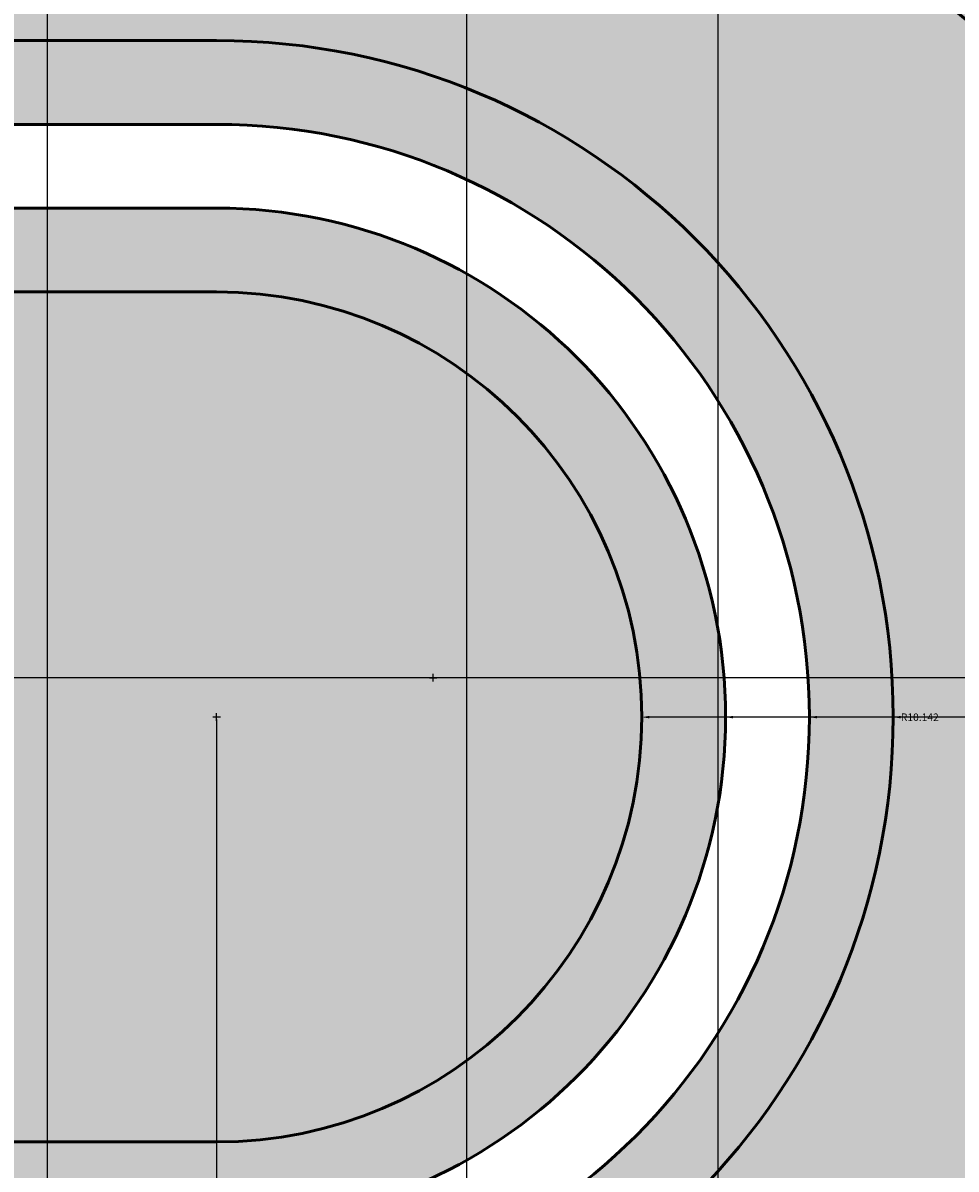
# Model space of a CAD drawing. Units: inches. Extents: x -12 to 334, y -10 to 186.
# Tile 54 of 77: x 222 to 244, y 69 to 96. Entities that reach past the tile are written whole.
import ezdxf

# ---------------------------------------------------------------- set-up
doc = ezdxf.new("R2010")
doc.units = ezdxf.units.IN
doc.header["$MEASUREMENT"] = 0
for name, color, linetype, lineweight in [('M-DIMS', 2, 'Continuous', 18), ('M-EQPM', 7, 'Continuous', 50), ('M-EQPM-PATT', 8, 'Continuous', 18)]:
    doc.layers.add(name, color=color, linetype=linetype, lineweight=lineweight)
doc.styles.get("Standard").update_dxf_attribs({"font": 'arial.ttf'})
doc.dimstyles.get("Standard").update_dxf_attribs({"dimtxt": 0.18, "dimasz": 0.18, "dimexe": 0.18, "dimexo": 0.0625, "dimgap": 0.09, "dimtad": 0, "dimtih": 1, "dimtoh": 1, "dimdec": 4, "dimzin": 0, "dimdsep": 46, "dimtxsty": 'Standard', "dimcen": 0.09, "dimadec": 0, "dimazin": 0, "dimtfac": 1, "dimtdec": 4, "dimtofl": 0, "dimtmove": 0, "dimatfit": 3, "dimfxl": 1, "dimtolj": 1, "dimtzin": 0, "dimarcsym": 0})

# ---------------------------------------------------------------- blocks, each defined once
blk = doc.blocks.new('*D1')
at = {"layer": 'Defpoints', "color": 0, "transparency": 16777216}
for p in [(281.426, 91.899), (3.376, 80.692), (281.426, 14.304)]:
    blk.add_point(p, dxfattribs=at)
at = {"layer": 'M-DIMS', "color": 0, "lineweight": -2, "transparency": 16777216}
for p, q in [((281.426, 91.836), (281.426, 14.124)), ((3.376, 80.629), (3.376, 14.124)), ((3.556, 14.304), (141.935, 14.304)), ((281.246, 14.304), (142.867, 14.304))]:
    blk.add_line(p, q, dxfattribs=at)
at = {"layer": 'M-DIMS', "color": 0, "transparency": 16777216}
for points in [[(3.556, 14.334), (3.556, 14.274), (3.376, 14.304)], [(281.246, 14.334), (281.246, 14.274), (281.426, 14.304)]]:
    blk.add_solid(points, dxfattribs=at)
at = {"layer": 'M-DIMS', "color": 0, "transparency": 16777216, "insert": (142.401, 14.304), "char_height": 0.18, "attachment_point": 5}
blk.add_mtext('\\A1;278.05', dxfattribs=at)
blk = doc.blocks.new('*D17')
at = {"layer": 'Defpoints', "color": 0, "transparency": 16777216}
for p in [(106.177, 102.896), (105.892, 56.321), (295.976, 56.321)]:
    blk.add_point(p, dxfattribs=at)
at = {"layer": 'M-DIMS', "color": 0, "lineweight": -2, "transparency": 16777216}
for p, q in [((106.24, 102.896), (296.156, 102.896)), ((295.976, 102.716), (295.976, 79.79)), ((295.976, 56.501), (295.976, 79.426)), ((105.954, 56.321), (296.156, 56.321))]:
    blk.add_line(p, q, dxfattribs=at)
at = {"layer": 'M-DIMS', "color": 0, "transparency": 16777216}
for points in [[(295.946, 102.716), (296.006, 102.716), (295.976, 102.896)], [(295.946, 56.501), (296.006, 56.501), (295.976, 56.321)]]:
    blk.add_solid(points, dxfattribs=at)
at = {"layer": 'M-DIMS', "color": 0, "transparency": 16777216, "insert": (295.976, 79.608), "char_height": 0.18, "attachment_point": 5}
blk.add_mtext('\\A1;46.575', dxfattribs=at)
blk = doc.blocks.new('*D27')
at = {"layer": 'Defpoints', "color": 0, "transparency": 16777216}
for p in [(238.576, 169.385), (216.576, 32.854), (238.576, 32.854)]:
    blk.add_point(p, dxfattribs=at)
at = {"layer": 'M-DIMS', "color": 0, "lineweight": -2, "transparency": 16777216}
for p, q in [((216.576, 32.917), (216.576, 169.565)), ((216.756, 169.385), (227.357, 169.385)), ((238.396, 169.385), (227.796, 169.385)), ((238.576, 32.917), (238.576, 169.565))]:
    blk.add_line(p, q, dxfattribs=at)
at = {"layer": 'M-DIMS', "color": 0, "transparency": 16777216}
for points in [[(216.756, 169.415), (216.756, 169.355), (216.576, 169.385)], [(238.396, 169.415), (238.396, 169.355), (238.576, 169.385)]]:
    blk.add_solid(points, dxfattribs=at)
at = {"layer": 'M-DIMS', "color": 0, "transparency": 16777216, "insert": (227.576, 169.385), "char_height": 0.18, "attachment_point": 5}
blk.add_mtext('\\A1;22', dxfattribs=at)
blk = doc.blocks.new('*D28')
at = {"layer": 'Defpoints', "color": 0, "transparency": 16777216}
for p in [(232.576, 169.385), (222.576, 30.854), (232.576, 30.854)]:
    blk.add_point(p, dxfattribs=at)
at = {"layer": 'M-DIMS', "color": 0, "lineweight": -2, "transparency": 16777216}
for p, q in [((222.576, 30.917), (222.576, 169.565)), ((222.756, 169.385), (227.366, 169.385)), ((232.396, 169.385), (227.786, 169.385)), ((232.576, 30.917), (232.576, 169.565))]:
    blk.add_line(p, q, dxfattribs=at)
at = {"layer": 'M-DIMS', "color": 0, "transparency": 16777216}
for points in [[(222.756, 169.415), (222.756, 169.355), (222.576, 169.385)], [(232.396, 169.415), (232.396, 169.355), (232.576, 169.385)]]:
    blk.add_solid(points, dxfattribs=at)
at = {"layer": 'M-DIMS', "color": 0, "transparency": 16777216, "insert": (227.576, 169.385), "char_height": 0.18, "attachment_point": 5}
blk.add_mtext('\\A1;10', dxfattribs=at)
blk = doc.blocks.new('*D33')
at = {"layer": 'Defpoints', "color": 0, "transparency": 16777216}
for p in [(226.608, 79.754), (216.428, 61.105), (226.608, 14.304)]:
    blk.add_point(p, dxfattribs=at)
at = {"layer": 'M-DIMS', "color": 0, "lineweight": -2, "transparency": 16777216}
for p, q in [((226.608, 79.692), (226.608, 14.124)), ((216.428, 61.042), (216.428, 14.124)), ((216.608, 14.304), (221.133, 14.304)), ((226.428, 14.304), (221.903, 14.304))]:
    blk.add_line(p, q, dxfattribs=at)
at = {"layer": 'M-DIMS', "color": 0, "transparency": 16777216}
for points in [[(216.608, 14.334), (216.608, 14.274), (216.428, 14.304)], [(226.428, 14.334), (226.428, 14.274), (226.608, 14.304)]]:
    blk.add_solid(points, dxfattribs=at)
at = {"layer": 'M-DIMS', "color": 0, "transparency": 16777216, "insert": (221.518, 14.304), "char_height": 0.18, "attachment_point": 5}
blk.add_mtext('\\A1;10.18', dxfattribs=at)
blk = doc.blocks.new('*D37')
at = {"layer": 'Defpoints', "color": 0, "transparency": 16777216}
for p in [(245.935, 169.385), (232.576, 46.854), (245.935, 46.854)]:
    blk.add_point(p, dxfattribs=at)
at = {"layer": 'M-DIMS', "color": 0, "lineweight": -2, "transparency": 16777216}
for p, q in [((232.576, 46.917), (232.576, 169.565)), ((232.756, 169.385), (238.871, 169.385)), ((245.755, 169.385), (239.641, 169.385)), ((245.935, 46.917), (245.935, 169.565))]:
    blk.add_line(p, q, dxfattribs=at)
at = {"layer": 'M-DIMS', "color": 0, "transparency": 16777216}
for points in [[(232.756, 169.415), (232.756, 169.355), (232.576, 169.385)], [(245.755, 169.415), (245.755, 169.355), (245.935, 169.385)]]:
    blk.add_solid(points, dxfattribs=at)
at = {"layer": 'M-DIMS', "color": 0, "transparency": 16777216, "insert": (239.256, 169.385), "char_height": 0.18, "attachment_point": 5}
blk.add_mtext('\\A1;13.36', dxfattribs=at)
blk = doc.blocks.new('*D39')
at = {"layer": 'Defpoints', "color": 0, "transparency": 16777216}
for p in [(279.726, 80.692), (-11.174, 45.854), (269.381, 45.854)]:
    blk.add_point(p, dxfattribs=at)
at = {"layer": 'M-DIMS', "color": 0, "lineweight": -2, "transparency": 16777216}
for p, q in [((279.664, 80.692), (-11.354, 80.692)), ((-11.174, 80.512), (-11.174, 63.455)), ((-11.174, 46.034), (-11.174, 63.091)), ((269.318, 45.854), (-11.354, 45.854))]:
    blk.add_line(p, q, dxfattribs=at)
at = {"layer": 'M-DIMS', "color": 0, "transparency": 16777216}
for points in [[(-11.204, 80.512), (-11.144, 80.512), (-11.174, 80.692)], [(-11.204, 46.034), (-11.144, 46.034), (-11.174, 45.854)]]:
    blk.add_solid(points, dxfattribs=at)
at = {"layer": 'M-DIMS', "color": 0, "transparency": 16777216, "insert": (-11.174, 63.273), "char_height": 0.18, "attachment_point": 5}
blk.add_mtext('\\A1;34.84', dxfattribs=at)
blk = doc.blocks.new('*D40')
at = {"layer": 'Defpoints', "color": 0, "transparency": 16777216}
for p in [(278.229, 116.208), (187.394, 91.899)]:
    blk.add_point(p, dxfattribs=at)
at = {"layer": 'M-DIMS', "color": 0, "lineweight": -2, "transparency": 16777216}
for p, q in [((332.73, 130.793), (278.403, 116.254)), ((187.394, 91.809), (187.394, 91.989)), ((187.304, 91.899), (187.484, 91.899))]:
    blk.add_line(p, q, dxfattribs=at)
at = {"layer": 'M-DIMS', "color": 0, "transparency": 16777216}
blk.add_solid([(278.395, 116.283), (278.411, 116.225), (278.229, 116.208)], dxfattribs=at)
at = {"layer": 'M-DIMS', "color": 0, "transparency": 16777216, "insert": (333.21, 130.793), "char_height": 0.18, "attachment_point": 5}
blk.add_mtext('\\A1;R94.03', dxfattribs=at)
blk = doc.blocks.new('*D41')
at = {"layer": 'Defpoints', "color": 0, "transparency": 16777216}
for p in [(190.169, 91.899), (277.343, 68.515)]:
    blk.add_point(p, dxfattribs=at)
at = {"layer": 'M-DIMS', "color": 0, "lineweight": -2, "transparency": 16777216}
for p, q in [((190.169, 91.809), (190.169, 91.989)), ((190.079, 91.899), (190.259, 91.899)), ((329.648, 54.485), (277.517, 68.469)), ((329.828, 54.485), (329.648, 54.485))]:
    blk.add_line(p, q, dxfattribs=at)
at = {"layer": 'M-DIMS', "color": 0, "transparency": 16777216}
blk.add_solid([(277.525, 68.498), (277.509, 68.44), (277.343, 68.515)], dxfattribs=at)
at = {"layer": 'M-DIMS', "color": 0, "transparency": 16777216, "insert": (330.307, 54.485), "char_height": 0.18, "attachment_point": 5}
blk.add_mtext('\\A1;R90.26', dxfattribs=at)
blk = doc.blocks.new('*D43')
at = {"layer": 'Defpoints', "color": 0, "transparency": 16777216}
for p in [(246.06, 94.98), (231.776, 80.692)]:
    blk.add_point(p, dxfattribs=at)
at = {"layer": 'M-DIMS', "color": 0, "lineweight": -2, "transparency": 16777216}
for p, q in [((254.631, 103.553), (246.187, 95.108)), ((254.811, 103.553), (254.631, 103.553)), ((231.686, 80.692), (231.866, 80.692)), ((231.776, 80.602), (231.776, 80.782))]:
    blk.add_line(p, q, dxfattribs=at)
at = {"layer": 'M-DIMS', "color": 0, "transparency": 16777216}
blk.add_solid([(246.166, 95.129), (246.209, 95.086), (246.06, 94.98)], dxfattribs=at)
at = {"layer": 'M-DIMS', "color": 0, "transparency": 16777216, "insert": (255.36, 103.553), "char_height": 0.18, "attachment_point": 5}
blk.add_mtext('\\A1;R20.204', dxfattribs=at)
blk = doc.blocks.new('*D45')
at = {"layer": 'Defpoints', "color": 0, "transparency": 16777216}
for p in [(226.608, 79.754), (242.751, 79.75)]:
    blk.add_point(p, dxfattribs=at)
at = {"layer": 'M-DIMS', "color": 0, "lineweight": -2, "transparency": 16777216}
for p, q in [((226.518, 79.754), (226.698, 79.754)), ((226.608, 79.664), (226.608, 79.844)), ((252.436, 79.748), (242.931, 79.75))]:
    blk.add_line(p, q, dxfattribs=at)
at = {"layer": 'M-DIMS', "color": 0, "transparency": 16777216}
blk.add_solid([(242.931, 79.78), (242.931, 79.72), (242.751, 79.75)], dxfattribs=at)
at = {"layer": 'M-DIMS', "color": 0, "transparency": 16777216, "insert": (252.985, 79.748), "char_height": 0.18, "attachment_point": 5}
blk.add_mtext('\\A1;R16.142', dxfattribs=at)
blk = doc.blocks.new('*D46')
at = {"layer": 'Defpoints', "color": 0, "transparency": 16777216}
for p in [(226.608, 79.754), (240.751, 79.75)]:
    blk.add_point(p, dxfattribs=at)
at = {"layer": 'M-DIMS', "color": 0, "lineweight": -2, "transparency": 16777216}
for p, q in [((226.518, 79.754), (226.698, 79.754)), ((226.608, 79.664), (226.608, 79.844)), ((249.236, 79.748), (240.931, 79.75))]:
    blk.add_line(p, q, dxfattribs=at)
at = {"layer": 'M-DIMS', "color": 0, "transparency": 16777216}
blk.add_solid([(240.931, 79.78), (240.931, 79.72), (240.751, 79.75)], dxfattribs=at)
at = {"layer": 'M-DIMS', "color": 0, "transparency": 16777216, "insert": (249.785, 79.748), "char_height": 0.18, "attachment_point": 5}
blk.add_mtext('\\A1;R14.142', dxfattribs=at)
blk = doc.blocks.new('*D47')
at = {"layer": 'Defpoints', "color": 0, "transparency": 16777216}
for p in [(226.608, 79.754), (238.751, 79.75)]:
    blk.add_point(p, dxfattribs=at)
at = {"layer": 'M-DIMS', "color": 0, "lineweight": -2, "transparency": 16777216}
for p, q in [((226.518, 79.754), (226.698, 79.754)), ((226.608, 79.664), (226.608, 79.844)), ((246.036, 79.748), (238.931, 79.75))]:
    blk.add_line(p, q, dxfattribs=at)
at = {"layer": 'M-DIMS', "color": 0, "transparency": 16777216}
blk.add_solid([(238.931, 79.78), (238.931, 79.72), (238.751, 79.75)], dxfattribs=at)
at = {"layer": 'M-DIMS', "color": 0, "transparency": 16777216, "insert": (246.585, 79.748), "char_height": 0.18, "attachment_point": 5}
blk.add_mtext('\\A1;R12.142', dxfattribs=at)
blk = doc.blocks.new('*D48')
at = {"layer": 'Defpoints', "color": 0, "transparency": 16777216}
for p in [(226.608, 79.754), (236.751, 79.75)]:
    blk.add_point(p, dxfattribs=at)
at = {"layer": 'M-DIMS', "color": 0, "lineweight": -2, "transparency": 16777216}
for p, q in [((226.518, 79.754), (226.698, 79.754)), ((226.608, 79.664), (226.608, 79.844)), ((242.836, 79.748), (236.931, 79.75))]:
    blk.add_line(p, q, dxfattribs=at)
at = {"layer": 'M-DIMS', "color": 0, "transparency": 16777216}
blk.add_solid([(236.931, 79.78), (236.931, 79.72), (236.751, 79.75)], dxfattribs=at)
at = {"layer": 'M-DIMS', "color": 0, "transparency": 16777216, "insert": (243.385, 79.748), "char_height": 0.18, "attachment_point": 5}
blk.add_mtext('\\A1;R10.142', dxfattribs=at)

msp = doc.modelspace()

# ---------------------------------------------------------------- hatches: boundary and pattern name
at = {"layer": 'M-EQPM-PATT', "transparency": 33554556}
h = msp.add_hatch(color=256, dxfattribs=at)
h.set_gradient(color1=(248, 206, 179), color2=(248, 206, 179), tint=1)
h.paths.add_polyline_path([(179.7818, 136.8871), (126.9567, 136.8871), (106.1771, 100.8958), (171.5458, 100.8958)])
h.paths.add_polyline_path([(268.3808, 136.9435), (214.0166, 136.9435), (214.0166, 154.8345), (196.3421, 154.8345), (196.3421, 136.8871), (179.7818, 136.8871), (171.5458, 100.8958), (231.7758, 100.8958, -0.4142136), (251.9801, 80.6915), (279.7263, 80.6915, 0.1631825)])
at = {"layer": 'M-EQPM-PATT'}
h = msp.add_hatch(color=256, dxfattribs=at)
h.set_gradient(color1=(205, 32, 39), color2=(205, 32, 39), tint=1)
h.paths.add_polyline_path([(64.5, 80.754), (64.5, 89.8963), (226.6083, 89.8963, -1), (226.6083, 69.6117), (64.5, 69.6117), (64.5, 78.754), (4.4744, 78.754, 0.384914), (23.5807, 61.4872), (37.1002, 61.4872), (37.1002, 33.6752), (53.1002, 33.6752), (53.1002, 61.4872), (64.5, 61.4872), (64.5, 63.6117), (226.6083, 63.6117, 1), (226.6083, 95.8963), (64.5, 95.8963), (64.5, 99.8958), (53.1002, 99.8958), (53.1002, 127.7078), (37.1002, 127.7078), (37.1002, 99.8958), (23.5807, 99.8958, 0.4132606), (4.3766, 80.754)])
h.paths.add_polyline_path([(64.5, 91.8963), (64.5, 93.8963), (226.6083, 93.8963, -1), (226.6083, 65.6117), (64.5, 65.6117), (64.5, 67.6117), (226.6083, 67.6117, 1), (226.6083, 91.8963)], flags=16)
h = msp.add_hatch(color=256, dxfattribs=at)
h.set_gradient(color1=(94, 103, 175), color2=(94, 103, 175), tint=1)
h.paths.add_polyline_path([(129.093, 89.8963), (86.8879, 89.8963), (86.8879, 69.6117), (129.093, 69.6117)], flags=17)
h.paths.add_polyline_path([(170.9079, 89.8963), (130.8573, 89.8963), (130.8573, 69.6117), (170.9079, 69.6117)], flags=17)
h.paths.add_polyline_path([(216.4278, 89.8963), (172.6722, 89.8963), (172.6722, 69.6117), (216.4278, 69.6117)], flags=17)
h.paths.add_polyline_path([(245.9354, 82.6969), (247.9354, 82.6969), (247.9354, 46.8541), (268.3808, 46.8541, 0.0998398), (279.7263, 80.6915), (251.9801, 80.6915, 0.4142136), (231.7758, 100.8958), (84.7229, 100.8958), (84.7229, 109.0583), (83.7229, 109.0583), (83.7229, 95.8963), (129.093, 95.8963), (129.093, 98.1081), (130.8573, 98.1081), (130.8573, 95.8963), (170.9079, 95.8963), (170.9079, 98.1081), (172.6722, 98.1081), (172.6722, 95.8963), (216.4278, 95.8963), (216.4278, 98.1081), (218.1922, 98.1081), (218.1922, 95.8963), (226.6083, 95.8963, -1), (226.6083, 63.6117), (218.1922, 63.6117), (218.1922, 61.1045), (216.4278, 61.1045), (216.4278, 63.6117), (172.6722, 63.6117), (172.6722, 61.1045), (170.9079, 61.1045), (170.9079, 63.6117), (130.8573, 63.6117), (130.8573, 61.1045), (129.093, 61.1045), (129.093, 63.6117), (87.8879, 63.6117), (87.8879, 56.3205), (105.8919, 56.3205), (105.8919, 28.8541), (115.8919, 28.8541), (115.8919, 46.8541), (222.5761, 46.8541), (222.5761, 30.8541), (232.5761, 30.8541), (232.5761, 46.8541), (245.9354, 46.8541)])
h.paths.add_polyline_path([(86.8879, 89.8963), (75.9244, 89.8963), (75.9244, 69.6117), (86.8879, 69.6117)])
h.paths.add_polyline_path([(83.7229, 109.0583), (75.9244, 109.0583), (75.9244, 95.8963), (83.7229, 95.8963)])
h.paths.add_polyline_path([(226.6083, 89.8963), (218.1922, 89.8963), (218.1922, 69.6117), (226.6083, 69.6117, 1)], flags=17)
h = msp.add_hatch(color=256, dxfattribs=at)
h.set_gradient(color1=(0, 0, 255), color2=(0, 0, 255), tint=1)
h.paths.add_polyline_path([(84.7229, 100.8958), (84.7229, 109.0583), (83.7229, 109.0583), (83.7229, 95.8963), (129.093, 95.8963), (129.093, 98.1081), (130.8573, 98.1081), (130.8573, 95.8963), (170.9079, 95.8963), (170.9079, 98.1081), (172.6722, 98.1081), (172.6722, 95.8963), (216.4278, 95.8963), (216.4278, 98.1081), (218.1922, 98.1081), (218.1922, 95.8963), (226.6083, 95.8963, -1), (226.6083, 63.6117), (218.1922, 63.6117), (218.1922, 61.1045), (216.4278, 61.1045), (216.4278, 63.6117), (172.6722, 63.6117), (172.6722, 61.1045), (170.9079, 61.1045), (170.9079, 63.6117), (130.8573, 63.6117), (130.8573, 61.1045), (129.093, 61.1045), (129.093, 63.6117), (87.8879, 63.6117), (87.8879, 56.3205), (105.8919, 56.3205), (105.8919, 28.8541), (115.8919, 28.8541), (115.8919, 46.8541), (222.5761, 46.8541), (222.5761, 30.8541), (232.5761, 30.8541), (232.5761, 46.8541), (245.9354, 46.8541), (245.9354, 82.6969), (247.9354, 82.6969), (247.9354, 46.8541), (268.3808, 46.8541, 0.0998398), (279.7263, 80.6915), (251.9801, 80.6915, 0.4142136), (231.7758, 100.8958)])

# ---------------------------------------------------------------- linework, layer by layer
at = {"layer": 'M-EQPM'}
for points in [[(64.5, 63.6117), (226.6083, 63.6117, 1), (226.6083, 95.8963), (64.5, 95.8963)], [(64.5, 65.6117), (226.6083, 65.6117, 1), (226.6083, 93.8963), (64.5, 93.8963)], [(64.5, 67.6117), (226.6083, 67.6117, 1), (226.6083, 91.8963), (64.5, 91.8963)], [(64.5, 69.6117), (226.6083, 69.6117, 1), (226.6083, 89.8963), (64.5, 89.8963)]]:
    msp.add_lwpolyline(points, format="xyb", dxfattribs=at)
msp.add_arc((231.7758, 80.6915), 20.2043, 0, 90, dxfattribs=at)

# ---------------------------------------------------------------- dimensions: what is measured, and where the dimension line sits
at = {"layer": 'M-DIMS'}
for base, p1, p2, override, picture, middle in [((238.5761, 169.3845), (216.5761, 32.8541), (238.5761, 32.8541), {"dimdec": 0, "dimlfac": 1, "dimrnd": 0, "dimzin": 0, "dimdsep": 46, "dimlunit": 2}, '*D27', (227.5761, 169.3845)), ((232.5761, 169.3845), (222.5761, 30.8541), (232.5761, 30.8541), {"dimdec": 0, "dimlfac": 1, "dimrnd": 0, "dimzin": 0, "dimdsep": 46, "dimlunit": 2}, '*D28', (227.5761, 169.3845)), ((245.9354, 169.3845), (232.5761, 46.8541), (245.9354, 46.8541), {"dimdec": 2, "dimlfac": 1, "dimrnd": 0, "dimzin": 0, "dimdsep": 46, "dimlunit": 2}, '*D37', (239.2558, 169.3845)), ((281.4256, 14.3041), (3.3765, 80.6915), (281.4256, 91.8988), {"dimdec": 2, "dimlfac": 1, "dimrnd": 0, "dimzin": 0, "dimdsep": 46, "dimlunit": 2}, '*D1', (142.401, 14.3041)), ((226.6083, 14.3041), (216.4278, 61.1045), (226.6083, 79.754), {"dimdec": 2, "dimlfac": 1, "dimrnd": 0, "dimzin": 0, "dimdsep": 46, "dimlunit": 2}, '*D33', (221.5181, 14.3041))]:
    dim = msp.add_linear_dim(base=base, p1=p1, p2=p2, dimstyle='Standard', override=override, dxfattribs=at)
    dim.commit()
    dim.dimension.update_dxf_attribs({"geometry": picture, "text_midpoint": middle})
for center, mpoint, override, picture, middle in [((187.3936, 91.8988), (278.2291, 116.2078), {"dimdec": 2, "dimlfac": 1, "dimrnd": 0, "dimzin": 0, "dimdsep": 46, "dimlunit": 2}, '*D40', (332.7304, 130.7932)), ((231.7758, 80.6915), (246.0602, 94.9802), {"dimdec": 3, "dimlfac": 1, "dimrnd": 0, "dimzin": 0, "dimdsep": 46, "dimlunit": 2}, '*D43', (255.3603, 103.5535)), ((190.1689, 91.8988), (277.3431, 68.5153), {"dimdec": 2, "dimlfac": 1, "dimrnd": 0, "dimzin": 0, "dimdsep": 46, "dimlunit": 2}, '*D41', (330.3074, 54.4851)), ((226.6083, 79.754), (242.7506, 79.75), {"dimdec": 3, "dimlfac": 1, "dimrnd": 0, "dimzin": 0, "dimdsep": 46, "dimlunit": 2}, '*D45', (252.436, 79.7476)), ((226.6083, 79.754), (240.7506, 79.75), {"dimdec": 3, "dimlfac": 1, "dimrnd": 0, "dimzin": 0, "dimdsep": 46, "dimlunit": 2}, '*D46', (249.236, 79.7476)), ((226.6083, 79.754), (238.7506, 79.75), {"dimdec": 3, "dimlfac": 1, "dimrnd": 0, "dimzin": 0, "dimdsep": 46, "dimlunit": 2}, '*D47', (246.036, 79.7476)), ((226.6083, 79.754), (236.7506, 79.75), {"dimdec": 3, "dimlfac": 1, "dimrnd": 0, "dimzin": 0, "dimdsep": 46, "dimlunit": 2}, '*D48', (242.836, 79.7476))]:
    dim = msp.add_radius_dim(center=center, mpoint=mpoint, dimstyle='Standard', override=override, dxfattribs=at)
    dim.commit()
    dim.dimension.update_dxf_attribs({"geometry": picture, "text_midpoint": middle, "dimtype": 164})
for base, p1, p2, override, picture, middle in [((295.9756, 56.3205), (106.1771, 102.8958), (105.8919, 56.3205), {"dimdec": 3, "dimlfac": 1, "dimrnd": 0, "dimzin": 0, "dimdsep": 46, "dimlunit": 2}, '*D17', (295.9756, 79.6082)), ((-11.1736, 45.8541), (279.7263, 80.6915), (269.3808, 45.8541), {"dimdec": 2, "dimlfac": 1, "dimrnd": 0, "dimzin": 0, "dimdsep": 46, "dimlunit": 2}, '*D39', (-11.1735, 63.2728))]:
    dim = msp.add_linear_dim(base=base, p1=p1, p2=p2, angle=90, dimstyle='Standard', override=override, dxfattribs=at)
    dim.commit()
    dim.dimension.update_dxf_attribs({"geometry": picture, "text_midpoint": middle})

doc.saveas('drawing.dxf')
